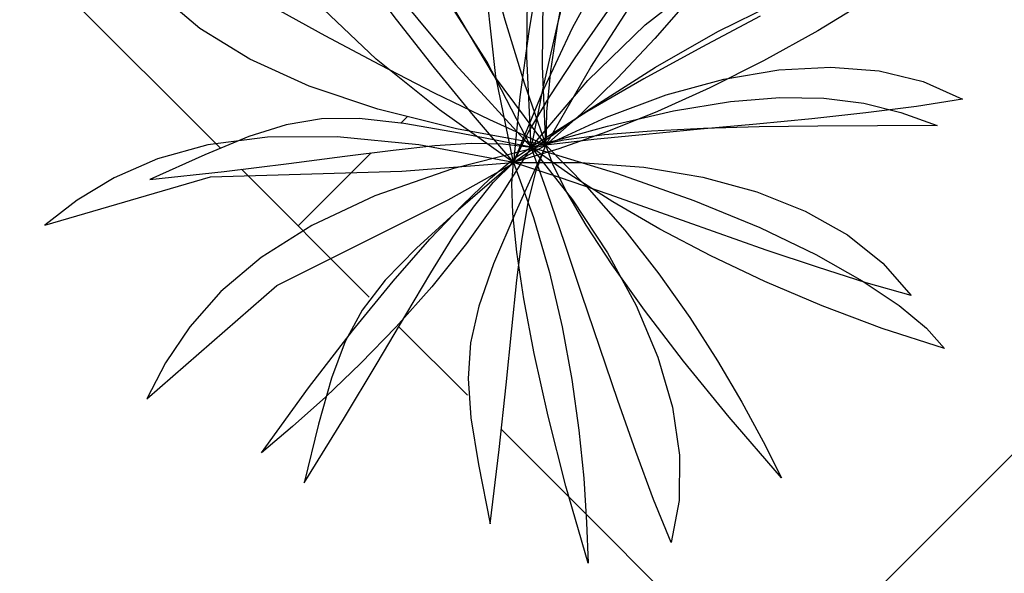
# Model space of a CAD drawing. Units: inches. Extents: x 3590 to 5167, y 65 to 1917.
# Tile 39 of 100: x 5035 to 5065, y 1340 to 1357. Entities that reach past the tile are written whole.
import ezdxf

# ---------------------------------------------------------------- set-up
doc = ezdxf.new("R2010")
doc.units = ezdxf.units.IN
doc.layers.add('A-FLOR-PATT', color=8, linetype='Continuous', lineweight=13)
doc.layers.add('L-PLNT', color=94, linetype='Continuous', lineweight=18)
doc.layers.add('DIENHOA', color=3, linetype='Continuous')

# ---------------------------------------------------------------- blocks, each defined once
blk = doc.blocks.new('Cay03_mb')
at = {"layer": 'DIENHOA'}
for p, q in [((-240.2, 277.8), (-88.4, 94.9)), ((55.7, 216.3), (37.3, 142.1)), ((0.2, 104.9), (1.6, 205.7)), ((147, 144.1), (218.5, 199.8)), ((-49.6, 98.5), (-104.2, 184.4)), ((290.2, 154.9), (217.4, 116.6)), ((37.3, 142.1), (20.5, 67.6)), ((75.9, 75.2), (147, 144.1)), ((217.4, 116.6), (145.5, 77.3)), ((5.4, -7.8), (-49.6, 98.5)), ((5.4, -7.8), (0.2, 104.9)), ((-88.4, 94.9), (5.4, -7.8)), ((5.4, -7.8), (75.9, 75.2)), ((145.5, 77.3), (74.7, 36.1)), ((20.5, 67.6), (5.4, -7.8)), ((182.2, 37.2), (253, 48.9)), ((253, 48.9), (314.6, 54.1)), ((314.6, 54.1), (369.2, 53.3)), ((369.2, 53.3), (418.6, 46.8)), ((100.3, 18.4), (182.2, 37.2)), ((418.6, 46.8), (464.9, 35.2)), ((-254.7, 27.4), (-298.6, 20.1)), ((-208, 27.8), (-254.7, 27.4)), ((-152.7, 21.7), (-208, 27.8)), ((74.7, 36.1), (5.4, -7.8)), ((464.9, 35.2), (510, 19)), ((-298.6, 20.1), (-345, 5.4)), ((-83.4, 9.7), (-152.7, 21.7)), ((5.4, -7.8), (100.3, 18.4)), ((219.6, 15.4), (155, 12.2)), ((289, 17.4), (219.6, 15.4)), ((361.6, 18.5), (289, 17.4)), ((435.8, 18.9), (361.6, 18.5)), ((510, 19), (435.8, 18.9)), ((-345, 5.4), (-399.6, -17.1)), ((5.4, -7.8), (-83.4, 9.7)), ((46.3, 0.9), (5.4, -7.8)), ((96.7, 7.5), (46.3, 0.9)), ((155, 12.2), (96.7, 7.5)), ((-225.8, -18.9), (-165.8, -11.3)), ((-165.8, -11.3), (-114, -5.7)), ((-114, -5.7), (-69, -2.9)), ((-69, -2.9), (-29.6, -3.4)), ((5.4, -7.8), (-33.2, -69.5)), ((-29.6, -3.4), (5.4, -7.8)), ((-16.5, -22.4), (5.4, -7.8)), ((5.4, -7.8), (56.8, -73.3)), ((25.9, -64.4), (5.4, -7.8)), ((5.4, -7.8), (112.8, -40.3)), ((53.5, -41.6), (5.4, -7.8)), ((-399.6, -17.1), (-468, -47.9)), ((-295.3, -27.9), (-225.8, -18.9)), ((-45.1, -46.3), (-16.5, -22.4)), ((-375.6, -37.8), (-295.3, -27.9)), ((-468, -47.9), (-375.6, -37.8)), ((-79.8, -79.6), (-45.1, -46.3)), ((107, -75.7), (53.5, -41.6)), ((112.8, -40.3), (207.5, -73.8)), ((-33.2, -69.5), (-74.6, -127.3)), ((47, -125.9), (25.9, -64.4)), ((56.8, -73.3), (100.4, -139.1)), ((-120.2, -122.1), (-79.8, -79.6)), ((165.5, -109.6), (107, -75.7)), ((207.5, -73.8), (289.5, -107.6)), ((228.7, -142.8), (165.5, -109.6)), ((289.5, -107.6), (359.3, -141.1)), ((-165.9, -174.1), (-120.2, -122.1)), ((-74.6, -127.3), (-117.8, -181.1)), ((68.7, -190.6), (47, -125.9)), ((100.4, -139.1), (135.9, -204.3)), ((296, -174.7), (228.7, -142.8)), ((359.3, -141.1), (416.9, -173.5)), ((-216.3, -235.6), (-165.9, -174.1)), ((-117.8, -181.1), (-162.1, -230.9)), ((367.1, -204.8), (296, -174.7)), ((416.9, -173.5), (462.6, -204.2)), ((90.8, -256.6), (68.7, -190.6)), ((135.9, -204.3), (162.8, -268.3)), ((441.6, -232.7), (367.1, -204.8)), ((462.6, -204.2), (496.5, -232.5)), ((-162.1, -230.9), (-206.3, -276.5)), ((-271, -306.6), (-216.3, -235.6)), ((518.9, -257.7), (441.6, -232.7)), ((496.5, -232.5), (518.9, -257.7)), ((113.1, -322.2), (90.8, -256.6)), ((162.8, -268.3), (181, -330.4)), ((-206.3, -276.5), (-249.6, -317.8)), ((-329.5, -387.1), (-271, -306.6)), ((-249.6, -317.8), (-291, -354.7)), ((135.4, -385.6), (113.1, -322.2)), ((181, -330.4), (190, -390)), ((-291, -354.7), (-329.5, -387.1)), ((157.6, -445), (135.4, -385.6)), ((190, -390), (189.6, -446.3)), ((179.5, -498.7), (157.6, -445)), ((189.6, -446.3), (179.5, -498.7))]:
    blk.add_line(p, q, dxfattribs=at)
for points in [[(23.7, -5.4), (-41, 82.2), (-91.8, 167.1), (-129.7, 249.5), (-155.6, 329.6), (-170.2, 407.8), (-174.7, 484.2), (-169.8, 559.3), (-156.5, 633.1)], [(-156.5, 633.1), (-132.5, 551.3), (-110.5, 470), (-89.8, 389.2), (-69.6, 309), (-49, 229.4), (-27.1, 150.4), (-3.2, 72.1), (23.7, -5.4)], [(-16.4, -26.7), (-38.3, 80), (-48.9, 178.3), (-48.7, 269), (-38.5, 352.6), (-19.1, 429.7), (9, 501), (44.9, 567.1), (87.9, 628.5)], [(87.9, 628.5), (75.5, 544.2), (61.3, 461.2), (46.1, 379.1), (30.8, 297.8), (16.1, 216.9), (2.9, 136), (-8.3, 54.9), (-16.4, -26.7)], [(23.7, -5.4), (19.8, 93), (20.3, 177), (25, 248.5), (34, 309.8), (47.3, 362.7), (64.9, 409.3), (86.8, 451.7), (112.9, 491.9)], [(112.9, 491.9), (96, 419.7), (79.5, 347.4), (63.9, 276.5), (50, 208.4), (38.4, 144.8), (29.7, 86.9), (24.6, 36.3), (23.7, -5.4)], [(-395.6, 473.7), (-347.5, 405.6), (-300.6, 339.5), (-254.3, 275.1), (-208.3, 212.3), (-161.9, 150.9), (-114.8, 90.7), (-66.5, 31.6), (-16.4, -26.7)], [(-16.4, -26.7), (-108.3, 38.6), (-186.9, 101.7), (-252.4, 163.5), (-305.1, 224.4), (-345.4, 285.2), (-373.7, 346.6), (-390.4, 409.2), (-395.6, 473.7)], [(384.3, 437.5), (342.2, 367.8), (298.1, 301.7), (252.6, 239.4), (206.1, 181.1), (159.4, 127.2), (113, 78), (67.6, 33.6), (23.7, -5.4)], [(23.7, -5.4), (79.9, 91.7), (134.1, 176.2), (185.8, 248.4), (234.3, 308.7), (279, 357.3), (319.3, 394.8), (354.6, 421.4), (384.3, 437.5)], [(273.2, 387.3), (227.6, 328.8), (182.3, 270.1), (138.4, 212.3), (97.2, 156.4), (60, 103.4), (27.8, 54.6), (1.9, 10.8), (-16.4, -26.7)], [(-16.4, -26.7), (21.4, 64.2), (57, 140.3), (91.4, 203.3), (125.2, 255.1), (159.5, 297.5), (195, 332.5), (232.7, 361.8), (273.2, 387.3)], [(-530.5, 289.7), (-458.3, 248.1), (-387.9, 207.8), (-318.9, 168.7), (-250.8, 131.1), (-182.9, 94.8), (-114.9, 59.9), (-46.2, 26.5), (23.7, -5.4)], [(23.7, -5.4), (-87.2, 15.2), (-185, 39.6), (-270.3, 68.2), (-343.7, 101.4), (-405.9, 139.7), (-457.3, 183.5), (-498.7, 233.4), (-530.5, 289.7)], [(496.7, 224), (429.4, 178.4), (361.6, 136.9), (294.1, 99.5), (227.5, 66.1), (162.4, 36.7), (99.7, 11.5), (39.8, -9.7), (-16.4, -26.7)], [(-16.4, -26.7), (75.4, 37.9), (160.1, 91.8), (237.3, 135.7), (306.6, 170), (367.6, 195.4), (419.9, 212.5), (463.1, 221.9), (496.7, 224)], [(23.7, -5.4), (99.3, 29.7), (173.2, 57.1), (244.8, 76.7), (313.3, 88.3), (377.9, 91.8), (437.9, 87), (492.7, 73.8), (541.4, 52)], [(541.4, 52), (484.1, 42.9), (421.2, 34.8), (354.4, 27.6), (285.4, 20.9), (216.1, 14.5), (148.2, 8.1), (83.5, 1.6), (23.7, -5.4)], [(-16.4, -26.7), (-134, -4.7), (-235.3, 5.3), (-322, 4.7), (-395.9, -5), (-458.7, -22.3), (-512.3, -45.7), (-558.2, -73.6), (-598.4, -104.7)], [(-471.9, -320.3), (-310.5, -179.3), (-97.7, -73.3), (23.7, -5.4)], [(23.7, -5.4), (-92.3, -34.8), (-188.4, -68.2), (-266.9, -105.1), (-329.9, -144.9), (-379.7, -187), (-418.5, -230.7), (-448.5, -275.3), (-471.9, -320.3)], [(23.7, -5.4), (-13.6, -87.9), (-41.1, -152.6), (-59.6, -205), (-69.9, -250.7), (-72.8, -295), (-69.2, -343.6), (-59.7, -401.9), (-45.3, -475.5)], [(-45.3, -475.5), (-34.1, -383.2), (-25.4, -302.8), (-18.3, -233.1), (-12, -172.9), (-5.6, -121.2), (2, -76.8), (11.4, -38.5), (23.7, -5.4)], [(316.5, -418.1), (251.4, -342.8), (194.8, -273.3), (146.5, -210.2), (106.3, -153.8), (74.1, -104.7), (49.7, -63.4), (32.9, -30.1), (23.7, -5.4)], [(23.7, -5.4), (74.9, -57.1), (121.8, -110.6), (164.3, -165), (202.7, -219.4), (237, -272.9), (267.3, -324.5), (293.7, -373.2), (316.5, -418.1)], [(-598.4, -104.7), (-392.7, -44.4), (-155, -37.4), (-16.4, -26.7)], [(-276.2, -424.4), (-227.3, -345.4), (-185.7, -276.1), (-150, -215.7), (-119.1, -163.8), (-91.5, -119.5), (-66, -82.3), (-41.4, -51.6), (-16.4, -26.7)], [(-16.4, -26.7), (-84.9, -86), (-137, -133.1), (-175.8, -173), (-204.3, -210), (-225.5, -249.1), (-242.5, -294.7), (-258.4, -351.6), (-276.2, -424.4)], [(76.2, -524.2), (48.8, -428.5), (26.6, -341.7), (9.2, -264.1), (-3.6, -196.1), (-12.3, -138), (-17.1, -90.2), (-18.3, -53), (-16.4, -26.7)], [(-16.4, -26.7), (66.9, -26.6), (145.6, -32.7), (218.8, -44.9), (285.8, -63.1), (345.9, -87.1), (398.4, -116.6), (442.6, -151.6), (477.6, -191.8)], [(477.6, -191.8), (421.8, -176), (361.3, -156.9), (297.6, -135.5), (232.2, -112.6), (166.6, -89.4), (102.3, -66.6), (40.8, -45.4), (-16.4, -26.7)], [(-16.4, -26.7), (8.5, -95.1), (28.5, -163.3), (44.3, -230.6), (56.3, -296.1), (65, -359), (70.9, -418.5), (74.5, -473.9), (76.2, -524.2)]]:
    blk.add_lwpolyline(points, dxfattribs=at)

msp = doc.modelspace()

# ---------------------------------------------------------------- hatches: boundary and pattern name
at = {"layer": 'A-FLOR-PATT', "transparency": 33554687}
h = msp.add_hatch(dxfattribs=at)
h.set_pattern_fill('AR-HBONE', color=256, scale=0.2)
h.set_pattern_definition([(45, (-588.972, 0), (0, 28.73682), [60.96, -20.32]), (135, (-574.604, 14.368), (3e-15, 28.73682), [60.96, -20.32])])
h.paths.add_polyline_path([(5071.274, 1796.999), (4933.274, 1796.999), (4933.274, 1753.999), (4962.774, 1753.999, -0.414214), (4928.774, 1719.999), (4933.274, 1718.999), (4933.274, 1334.999), (5071.274, 1334.999)])
h.paths.add_polyline_path([(4951.78, 1521.077), (4951.715, 1521.04), (4951.563, 1520.895)], flags=16)
h.paths.add_polyline_path([(4952.267, 1521.376), (4952.198, 1521.371), (4952.198, 1521.356)], flags=0)
h.paths.add_polyline_path([(4967.051, 1529.728), (4965.231, 1528.694), (4963.411, 1527.714), (4961.756, 1526.851), (4963.589, 1527.449), (4964.036, 1527.478), (4962.975, 1527.249), (4961.76, 1526.852), (4959.792, 1525.834), (4958.005, 1524.895), (4956.24, 1523.93), (4954.504, 1522.919), (4954.129, 1522.682), (4953.361, 1521.997), (4953.366, 1521.998), (4953.605, 1522.064), (4955.106, 1522.761), (4956.921, 1523.434), (4958.678, 1523.915), (4960.358, 1524.2), (4961.945, 1524.286), (4964.171, 1524.108), (4965.958, 1523.309), (4963.863, 1522.976), (4965.187, 1522.499), (4963.366, 1522.497), (4961.545, 1522.487), (4959.764, 1522.461), (4958.304, 1522.419), (4957.974, 1522.388), (4956.307, 1522.232), (4954.718, 1522.071), (4953.251, 1521.899), (4953.525, 1521.623), (4954.331, 1521.379), (4956.243, 1521.23), (4958.039, 1520.93), (4959.684, 1520.483), (4961.16, 1519.896), (4963.107, 1518.8), (4964.393, 1517.325), (4962.973, 1517.726), (4964.558, 1516.661), (4965.407, 1515.708), (4963.507, 1516.322), (4961.68, 1517.005), (4959.935, 1517.745), (4958.282, 1518.528), (4956.732, 1519.343), (4955.295, 1520.175), (4954.672, 1520.572), (4954.513, 1520.627), (4955.658, 1519.318), (4956.703, 1517.982), (4957.644, 1516.647), (4958.485, 1515.334), (4959.55, 1513.524), (4960.438, 1511.769), (4958.841, 1513.62), (4957.452, 1515.325), (4955.819, 1517.459), (4956.665, 1515.448), (4957.111, 1513.923), (4957.447, 1511.714), (4957.076, 1509.793), (4956.538, 1511.11), (4955.992, 1512.569), (4955.444, 1514.125), (4954.898, 1515.735), (4954.357, 1517.356), (4953.824, 1518.943), (4953.305, 1520.452), (4953.065, 1521.116), (4952.971, 1521.146), (4952.949, 1521.086), (4952.73, 1520.199), (4953.37, 1518.024), (4953.757, 1516.373), (4954.051, 1514.765), (4954.264, 1513.221), (4954.471, 1511.131), (4954.497, 1510.402), (4954.409, 1511.76), (4954.264, 1513.221), (4954.051, 1514.765), (4953.757, 1516.373), (4953.37, 1518.024), (4952.877, 1519.698), (4952.716, 1520.141), (4952.533, 1519.059), (4952.374, 1517.789), (4952.219, 1516.312), (4952.046, 1514.6), (4951.833, 1512.626), (4951.557, 1510.363), (4951.203, 1512.168), (4950.852, 1514.339), (4950.985, 1516.376), (4951.66, 1518.286), (4952.593, 1520.481), (4952.357, 1521.13), (4951.855, 1520.328), (4950.839, 1518.908), (4949.777, 1517.587), (4948.916, 1516.617), (4948.111, 1515.256), (4947.089, 1513.554), (4945.889, 1511.615), (4946.326, 1513.402), (4946.562, 1514.249), (4945.528, 1513.327), (4944.581, 1512.531), (4946.018, 1514.508), (4947.204, 1516.048), (4947.893, 1517.313), (4949.307, 1518.764), (4950.414, 1519.767), (4950.451, 1519.806), (4952.267, 1521.376), (4951.645, 1521.493), (4950.404, 1521.18), (4948.044, 1520.359), (4946.119, 1519.452), (4944.572, 1518.475), (4943.35, 1517.443), (4941.997, 1515.92), (4941.661, 1515.275), (4942.813, 1516.99), (4944.572, 1518.475), (4946.119, 1519.452), (4948.044, 1520.359), (4950.404, 1521.18), (4951.645, 1521.493), (4949.647, 1521.868), (4948.6, 1521.756), (4947.126, 1521.57), (4945.42, 1521.348), (4943.45, 1521.105), (4941.183, 1520.856), (4942.86, 1521.613), (4943.873, 1522.03), (4942.952, 1521.909), (4941.41, 1521.485), (4939.543, 1520.67), (4938.968, 1520.226), (4940.733, 1521.299), (4942.952, 1521.909), (4943.702, 1522.008), (4945.894, 1522.7), (4947.565, 1522.714), (4948.921, 1522.566), (4951.131, 1522.183), (4950.971, 1522.297), (4948.129, 1523.006), (4946.035, 1523.707), (4944.232, 1524.521), (4942.707, 1525.461), (4941.444, 1526.537), (4940.43, 1527.761), (4939.649, 1529.143), (4941.421, 1528.122), (4943.147, 1527.132), (4944.841, 1526.175), (4946.514, 1525.25), (4948.179, 1524.359), (4948.365, 1524.263), (4946.475, 1526.045), (4945.181, 1527.54), (4944.19, 1529.033), (4943.496, 1530.54), (4943.278, 1531.36), (4942.498, 1531.919), (4943.114, 1531.762), (4942.959, 1533.659), (4944.14, 1531.989), (4944.612, 1531.323), (4946.202, 1530.463), (4947.486, 1529.509), (4948.79, 1528.226), (4950.368, 1526.237), (4949.485, 1528.155), (4948.851, 1530.123), (4948.491, 1532.041), (4948.381, 1533.918), (4948.501, 1535.76), (4948.827, 1537.573), (4949.418, 1535.565), (4949.957, 1533.569), (4950.464, 1531.586), (4950.961, 1529.617), (4951.391, 1527.954), (4951.724, 1530.687), (4952.201, 1532.58), (4952.889, 1534.33), (4953.77, 1535.951), (4954.827, 1537.46), (4954.521, 1535.39), (4954.273, 1533.937), (4955.58, 1535.663), (4956.748, 1536.739), (4956.159, 1534.78), (4955.589, 1532.873), (4955.043, 1531.006), (4954.525, 1529.166), (4954.038, 1527.341), (4953.638, 1525.733), (4953.611, 1525.586), (4953.398, 1524.166), (4953.382, 1524.009), (4954.07, 1525.476), (4954.912, 1527.022), (4956.136, 1528.894), (4957.847, 1530.577), (4959.376, 1531.54), (4958.256, 1530.104), (4957.143, 1528.663), (4956.066, 1527.243), (4955.056, 1525.871), (4954.141, 1524.571), (4953.352, 1523.372), (4953.311, 1523.303), (4953.273, 1522.925), (4953.261, 1522.382), (4954.103, 1523.373), (4954.63, 1524.284), (4955.961, 1526.358), (4957.23, 1528.13), (4958.421, 1529.609), (4960.037, 1531.368), (4961.374, 1532.375), (4962.101, 1532.77), (4961.07, 1531.061), (4959.987, 1529.438), (4958.869, 1527.908), (4958.15, 1527.007), (4959.803, 1528.003), (4961.589, 1528.793), (4963.391, 1529.328), (4965.211, 1529.632)], flags=16)
h.paths.add_polyline_path([(4962.944, 1523.182), (4961.107, 1523.422), (4960.392, 1523.362), (4962.35, 1523.331)], flags=0)
h.paths.add_polyline_path([(5049.541, 1584.551), (5049.476, 1584.515), (5049.325, 1584.37)], flags=16)
h.paths.add_polyline_path([(5050.028, 1584.851), (5049.959, 1584.845), (5049.959, 1584.83)], flags=0)
h.paths.add_polyline_path([(5042.333, 1581.949), (5043.88, 1582.926), (5045.806, 1583.833), (5048.165, 1584.654), (5049.406, 1584.967), (5047.408, 1585.342), (5046.361, 1585.231), (5044.888, 1585.044), (5043.181, 1584.822), (5041.211, 1584.579), (5038.944, 1584.33), (5040.622, 1585.087), (5041.634, 1585.504), (5040.713, 1585.383), (5039.171, 1584.959), (5037.304, 1584.144), (5036.729, 1583.7), (5038.494, 1584.773), (5040.713, 1585.383), (5041.463, 1585.482), (5043.655, 1586.174), (5045.326, 1586.188), (5046.682, 1586.04), (5048.893, 1585.657), (5048.732, 1585.771), (5045.891, 1586.48), (5043.796, 1587.181), (5041.994, 1587.996), (5040.468, 1588.935), (5039.205, 1590.011), (5038.191, 1591.235), (5037.41, 1592.617), (5039.182, 1591.596), (5040.909, 1590.607), (5042.602, 1589.649), (5044.275, 1588.724), (5045.94, 1587.833), (5046.126, 1587.738), (5044.237, 1589.519), (5042.942, 1591.015), (5041.952, 1592.508), (5041.257, 1594.014), (5041.039, 1594.834), (5040.26, 1595.393), (5040.875, 1595.237), (5040.721, 1597.133), (5041.901, 1595.463), (5042.373, 1594.798), (5043.963, 1593.938), (5045.247, 1592.983), (5046.552, 1591.701), (5048.129, 1589.712), (5047.247, 1591.63), (5046.613, 1593.597), (5046.252, 1595.515), (5046.142, 1597.392), (5046.262, 1599.234), (5046.588, 1601.047), (5047.179, 1599.039), (5047.718, 1597.043), (5048.225, 1595.06), (5048.722, 1593.091), (5049.152, 1591.429), (5049.485, 1594.161), (5049.962, 1596.054), (5050.65, 1597.804), (5051.532, 1599.425), (5052.589, 1600.934), (5052.283, 1598.864), (5052.034, 1597.411), (5053.341, 1599.137), (5054.509, 1600.213), (5053.92, 1598.254), (5053.35, 1596.348), (5052.805, 1594.48), (5052.286, 1592.64), (5051.799, 1590.815), (5051.4, 1589.207), (5051.373, 1589.06), (5051.159, 1587.64), (5051.143, 1587.483), (5051.831, 1588.95), (5052.673, 1590.496), (5053.898, 1592.368), (5055.608, 1594.051), (5057.137, 1595.014), (5056.017, 1593.578), (5054.904, 1592.137), (5053.828, 1590.717), (5052.817, 1589.345), (5051.902, 1588.046), (5051.113, 1586.846), (5051.072, 1586.777), (5051.034, 1586.399), (5051.022, 1585.856), (5051.864, 1586.847), (5052.391, 1587.758), (5053.723, 1589.832), (5054.991, 1591.604), (5056.182, 1593.083), (5057.798, 1594.842), (5059.135, 1595.849), (5059.863, 1596.244), (5058.831, 1594.535), (5057.749, 1592.912), (5056.63, 1591.382), (5055.912, 1590.482), (5057.564, 1591.477), (5059.35, 1592.267), (5061.152, 1592.802), (5062.972, 1593.106), (5064.812, 1593.203), (5062.992, 1592.169), (5061.172, 1591.188), (5059.518, 1590.325), (5061.35, 1590.924), (5061.797, 1590.952), (5060.737, 1590.723), (5059.521, 1590.326), (5057.553, 1589.308), (5055.766, 1588.369), (5054.002, 1587.404), (5052.265, 1586.393), (5051.891, 1586.156), (5051.122, 1585.471), (5051.127, 1585.472), (5051.366, 1585.538), (5052.867, 1586.235), (5054.682, 1586.908), (5056.439, 1587.389), (5058.12, 1587.675), (5059.706, 1587.76), (5061.933, 1587.583), (5063.719, 1586.783), (5061.624, 1586.45), (5062.949, 1585.973), (5061.127, 1585.971), (5059.307, 1585.961), (5057.525, 1585.935), (5056.065, 1585.893), (5055.735, 1585.862), (5054.068, 1585.707), (5052.479, 1585.546), (5051.012, 1585.373), (5051.286, 1585.097), (5052.092, 1584.853), (5054.004, 1584.704), (5055.8, 1584.404), (5057.446, 1583.958), (5058.921, 1583.37), (5060.868, 1582.274), (5062.154, 1580.799), (5060.734, 1581.2), (5062.32, 1580.135), (5063.168, 1579.182), (5061.269, 1579.796), (5059.441, 1580.479), (5057.696, 1581.219), (5056.043, 1582.003), (5054.493, 1582.817), (5053.057, 1583.649), (5052.433, 1584.047), (5052.274, 1584.101), (5053.42, 1582.793), (5054.464, 1581.457), (5055.405, 1580.121), (5056.247, 1578.809), (5057.311, 1576.998), (5058.199, 1575.244), (5056.602, 1577.094), (5055.213, 1578.799), (5053.58, 1580.933), (5054.427, 1578.922), (5054.872, 1577.397), (5055.208, 1575.189), (5054.838, 1573.267), (5054.299, 1574.584), (5053.754, 1576.043), (5053.206, 1577.599), (5052.659, 1579.209), (5052.118, 1580.83), (5051.585, 1582.417), (5051.066, 1583.927), (5050.826, 1584.59), (5050.733, 1584.62), (5050.711, 1584.561), (5050.491, 1583.673), (5051.131, 1581.498), (5051.518, 1579.847), (5051.813, 1578.24), (5052.026, 1576.695), (5052.233, 1574.605), (5052.258, 1573.876), (5052.17, 1575.234), (5052.026, 1576.695), (5051.813, 1578.24), (5051.518, 1579.847), (5051.131, 1581.498), (5050.638, 1583.172), (5050.477, 1583.615), (5050.294, 1582.533), (5050.136, 1581.263), (5049.981, 1579.786), (5049.807, 1578.074), (5049.594, 1576.1), (5049.318, 1573.837), (5048.965, 1575.642), (5048.613, 1577.813), (5048.747, 1579.85), (5049.421, 1581.76), (5050.354, 1583.955), (5050.118, 1584.604), (5049.616, 1583.802), (5048.6, 1582.382), (5047.538, 1581.061), (5046.677, 1580.091), (5045.872, 1578.73), (5044.85, 1577.028), (5043.651, 1575.089), (5044.087, 1576.877), (5044.324, 1577.723), (5043.289, 1576.801), (5042.342, 1576.005), (5043.779, 1577.982), (5044.966, 1579.522), (5045.655, 1580.787), (5047.068, 1582.239), (5048.175, 1583.241), (5048.213, 1583.28), (5050.028, 1584.851), (5049.406, 1584.967), (5048.165, 1584.654), (5045.806, 1583.833), (5043.88, 1582.926), (5042.333, 1581.949), (5041.111, 1580.917), (5039.758, 1579.394), (5039.423, 1578.749), (5040.575, 1580.464)], flags=16)
h.paths.add_polyline_path([(4954.799, 1533.12), (4954.262, 1532.079), (4953.831, 1530.935), (4953.505, 1529.636), (4953.283, 1528.133), (4953.167, 1526.376), (4953.156, 1524.315), (4953.277, 1521.236), (4952.802, 1521.842), (4951.557, 1521.998), (4950.976, 1521.961), (4952.661, 1521.941), (4952.802, 1521.842), (4953.152, 1523.593), (4953.167, 1526.376), (4953.283, 1528.133), (4953.609, 1530.346), (4954.456, 1532.592)], flags=0)
h.paths.add_polyline_path([(5050.563, 1585.316), (5049.318, 1585.472), (5048.737, 1585.435), (5050.422, 1585.415), (5050.563, 1585.316), (5050.914, 1587.067), (5050.928, 1589.851), (5051.045, 1591.607), (5051.371, 1593.82), (5052.217, 1596.066), (5052.56, 1596.594), (5052.024, 1595.554), (5051.592, 1594.409), (5051.266, 1593.11), (5051.045, 1591.607), (5050.928, 1589.851), (5050.918, 1587.789), (5051.038, 1584.71)], flags=0)
h.paths.add_polyline_path([(5058.153, 1586.836), (5060.111, 1586.805), (5060.705, 1586.656), (5058.868, 1586.896)], flags=0)
h.paths.add_polyline_path([(5049.541, 1430.936), (5049.476, 1430.9), (5049.325, 1430.755)], flags=16)
h.paths.add_polyline_path([(5050.028, 1431.236), (5049.959, 1431.231), (5049.959, 1431.215)], flags=0)
h.paths.add_polyline_path([(5046.588, 1447.432), (5047.179, 1445.425), (5047.718, 1443.429), (5048.225, 1441.446), (5048.722, 1439.476), (5049.152, 1437.814), (5049.485, 1440.546), (5049.962, 1442.439), (5050.65, 1444.189), (5051.532, 1445.811), (5052.589, 1447.319), (5052.283, 1445.249), (5052.034, 1443.796), (5053.341, 1445.522), (5054.509, 1446.598), (5053.92, 1444.64), (5053.35, 1442.733), (5052.805, 1440.865), (5052.286, 1439.025), (5051.799, 1437.201), (5051.4, 1435.592), (5051.373, 1435.445), (5051.159, 1434.025), (5051.143, 1433.868), (5051.831, 1435.335), (5052.673, 1436.881), (5053.898, 1438.753), (5055.608, 1440.436), (5057.137, 1441.4), (5056.017, 1439.963), (5054.904, 1438.522), (5053.828, 1437.102), (5052.817, 1435.73), (5051.902, 1434.431), (5051.113, 1433.231), (5051.072, 1433.162), (5051.034, 1432.784), (5051.022, 1432.242), (5051.864, 1433.232), (5052.391, 1434.143), (5053.723, 1436.217), (5054.991, 1437.989), (5056.182, 1439.468), (5057.798, 1441.227), (5059.135, 1442.235), (5059.863, 1442.629), (5058.831, 1440.921), (5057.749, 1439.298), (5056.63, 1437.767), (5055.912, 1436.867), (5057.564, 1437.863), (5059.35, 1438.652), (5061.152, 1439.187), (5062.972, 1439.491), (5064.812, 1439.588), (5062.992, 1438.554), (5061.172, 1437.573), (5059.518, 1436.71), (5061.35, 1437.309), (5061.797, 1437.337), (5060.737, 1437.108), (5059.521, 1436.711), (5057.553, 1435.693), (5055.766, 1434.754), (5054.002, 1433.789), (5052.265, 1432.778), (5051.891, 1432.541), (5051.122, 1431.856), (5051.127, 1431.857), (5051.366, 1431.923), (5052.867, 1432.62), (5054.682, 1433.293), (5056.439, 1433.775), (5058.12, 1434.06), (5059.706, 1434.145), (5061.933, 1433.968), (5063.719, 1433.168), (5061.624, 1432.835), (5062.949, 1432.358), (5061.127, 1432.357), (5059.307, 1432.346), (5057.525, 1432.32), (5056.065, 1432.278), (5055.735, 1432.248), (5054.068, 1432.092), (5052.479, 1431.931), (5051.012, 1431.759), (5051.286, 1431.482), (5052.092, 1431.238), (5054.004, 1431.089), (5055.8, 1430.789), (5057.446, 1430.343), (5058.921, 1429.755), (5060.868, 1428.66), (5062.154, 1427.185), (5060.734, 1427.585), (5062.32, 1426.52), (5063.168, 1425.567), (5061.269, 1426.181), (5059.441, 1426.865), (5057.696, 1427.604), (5056.043, 1428.388), (5054.493, 1429.202), (5053.057, 1430.034), (5052.433, 1430.432), (5052.274, 1430.487), (5053.42, 1429.178), (5054.464, 1427.842), (5055.405, 1426.506), (5056.247, 1425.194), (5057.311, 1423.383), (5058.199, 1421.629), (5056.602, 1423.479), (5055.213, 1425.184), (5053.58, 1427.318), (5054.427, 1425.307), (5054.872, 1423.782), (5055.208, 1421.574), (5054.838, 1419.652), (5054.299, 1420.97), (5053.754, 1422.428), (5053.206, 1423.984), (5052.659, 1425.595), (5052.118, 1427.215), (5051.585, 1428.802), (5051.066, 1430.312), (5050.826, 1430.975), (5050.733, 1431.005), (5050.711, 1430.946), (5050.491, 1430.058), (5051.131, 1427.883), (5051.518, 1426.232), (5051.813, 1424.625), (5052.026, 1423.081), (5052.233, 1420.991), (5052.258, 1420.261), (5052.17, 1421.619), (5052.026, 1423.081), (5051.813, 1424.625), (5051.518, 1426.232), (5051.131, 1427.883), (5050.638, 1429.558), (5050.477, 1430.001), (5050.294, 1428.918), (5050.136, 1427.648), (5049.981, 1426.171), (5049.807, 1424.459), (5049.594, 1422.485), (5049.318, 1420.222), (5048.965, 1422.028), (5048.613, 1424.199), (5048.747, 1426.235), (5049.421, 1428.146), (5050.354, 1430.34), (5050.118, 1430.989), (5049.616, 1430.187), (5048.6, 1428.768), (5047.538, 1427.446), (5046.677, 1426.477), (5045.872, 1425.116), (5044.85, 1423.413), (5043.651, 1421.474), (5044.087, 1423.262), (5044.324, 1424.109), (5043.289, 1423.186), (5042.342, 1422.391), (5043.779, 1424.368), (5044.966, 1425.907), (5045.655, 1427.173), (5047.068, 1428.624), (5048.175, 1429.627), (5048.213, 1429.666), (5050.028, 1431.236), (5049.406, 1431.353), (5048.165, 1431.039), (5045.806, 1430.218), (5043.88, 1429.311), (5042.333, 1428.334), (5041.111, 1427.302), (5039.758, 1425.779), (5039.423, 1425.134), (5040.575, 1426.849), (5042.333, 1428.334), (5043.88, 1429.311), (5045.806, 1430.218), (5048.165, 1431.039), (5049.406, 1431.353), (5047.408, 1431.727), (5046.361, 1431.616), (5044.888, 1431.429), (5043.181, 1431.207), (5041.211, 1430.964), (5038.944, 1430.715), (5040.622, 1431.472), (5041.634, 1431.89), (5040.713, 1431.769), (5039.171, 1431.345), (5037.304, 1430.53), (5036.729, 1430.085), (5038.494, 1431.158), (5040.713, 1431.769), (5041.463, 1431.867), (5043.655, 1432.559), (5045.326, 1432.573), (5046.682, 1432.425), (5048.893, 1432.042), (5048.732, 1432.156), (5045.891, 1432.865), (5043.796, 1433.566), (5041.994, 1434.381), (5040.468, 1435.321), (5039.205, 1436.396), (5038.191, 1437.62), (5037.41, 1439.002), (5039.182, 1437.982), (5040.909, 1436.992), (5042.602, 1436.034), (5044.275, 1435.109), (5045.94, 1434.218), (5046.126, 1434.123), (5044.237, 1435.904), (5042.942, 1437.4), (5041.952, 1438.893), (5041.257, 1440.399), (5041.039, 1441.219), (5040.26, 1441.778), (5040.875, 1441.622), (5040.721, 1443.518), (5041.901, 1441.848), (5042.373, 1441.183), (5043.963, 1440.323), (5045.247, 1439.369), (5046.552, 1438.086), (5048.129, 1436.097), (5047.247, 1438.015), (5046.613, 1439.982), (5046.252, 1441.901), (5046.142, 1443.778), (5046.262, 1445.619)], flags=16)
h.paths.add_polyline_path([(5052.382, 1444.255), (5051.623, 1442.78), (5052.024, 1441.939), (5052.56, 1442.98)], flags=0)
h.paths.add_polyline_path([(5050.563, 1431.701), (5049.318, 1431.857), (5048.737, 1431.821), (5050.422, 1431.8)], flags=0)
h.paths.add_polyline_path([(5058.153, 1433.221), (5060.111, 1433.19), (5060.705, 1433.041), (5058.868, 1433.281)], flags=0)
h.paths.add_polyline_path([(5049.541, 1352.285), (5049.476, 1352.249), (5049.325, 1352.104)], flags=16)
h.paths.add_polyline_path([(5050.028, 1352.585), (5049.959, 1352.58), (5049.959, 1352.564)], flags=0)
h.paths.add_polyline_path([(5046.588, 1368.781), (5047.179, 1366.774), (5047.718, 1364.778), (5048.225, 1362.795), (5048.722, 1360.825), (5049.152, 1359.163), (5049.485, 1361.896), (5049.962, 1363.789), (5050.65, 1365.538), (5051.532, 1367.16), (5052.589, 1368.669), (5052.283, 1366.598), (5052.034, 1365.145), (5053.341, 1366.871), (5054.509, 1367.947), (5053.92, 1365.989), (5053.35, 1364.082), (5052.805, 1362.214), (5052.286, 1360.374), (5051.799, 1358.55), (5051.4, 1356.942), (5051.373, 1356.794), (5051.159, 1355.374), (5051.143, 1355.218), (5051.831, 1356.684), (5052.673, 1358.23), (5053.898, 1360.102), (5055.608, 1361.786), (5057.137, 1362.749), (5056.017, 1361.313), (5054.904, 1359.872), (5053.828, 1358.452), (5052.817, 1357.079), (5051.902, 1355.78), (5051.113, 1354.581), (5051.072, 1354.512), (5051.034, 1354.133), (5051.022, 1353.591), (5051.864, 1354.581), (5052.391, 1355.492), (5053.723, 1357.566), (5054.991, 1359.338), (5056.182, 1360.817), (5057.798, 1362.577), (5059.135, 1363.584), (5059.863, 1363.979), (5058.831, 1362.27), (5057.749, 1360.647), (5056.63, 1359.117), (5055.912, 1358.216), (5057.564, 1359.212), (5059.35, 1360.001), (5061.152, 1360.536), (5062.972, 1360.841), (5064.812, 1360.937), (5062.992, 1359.903), (5061.172, 1358.923), (5059.518, 1358.059), (5061.35, 1358.658), (5061.797, 1358.687), (5060.737, 1358.458), (5059.521, 1358.061), (5057.553, 1357.043), (5055.766, 1356.103), (5054.002, 1355.138), (5052.265, 1354.127), (5051.891, 1353.89), (5051.122, 1353.206), (5051.127, 1353.206), (5051.366, 1353.272), (5052.867, 1353.969), (5054.682, 1354.643), (5056.439, 1355.124), (5058.12, 1355.409), (5059.706, 1355.495), (5061.933, 1355.317), (5063.719, 1354.518), (5061.624, 1354.184), (5062.949, 1353.708), (5061.127, 1353.706), (5059.307, 1353.695), (5057.525, 1353.669), (5056.065, 1353.627), (5055.735, 1353.597), (5054.068, 1353.441), (5052.479, 1353.28), (5051.012, 1353.108), (5051.286, 1352.831), (5052.092, 1352.587), (5054.004, 1352.439), (5055.8, 1352.138), (5057.446, 1351.692), (5058.921, 1351.104), (5060.868, 1350.009), (5062.154, 1348.534), (5060.734, 1348.935), (5062.32, 1347.869), (5063.168, 1346.916), (5061.269, 1347.53), (5059.441, 1348.214), (5057.696, 1348.954), (5056.043, 1349.737), (5054.493, 1350.551), (5053.057, 1351.383), (5052.433, 1351.781), (5052.274, 1351.836), (5053.42, 1350.527), (5054.464, 1349.191), (5055.405, 1347.855), (5056.247, 1346.543), (5057.311, 1344.733), (5058.199, 1342.978), (5056.602, 1344.828), (5055.213, 1346.534), (5053.58, 1348.667), (5054.427, 1346.656), (5054.872, 1345.132), (5055.208, 1342.923), (5054.838, 1341.002), (5054.299, 1342.319), (5053.754, 1343.778), (5053.206, 1345.334), (5052.659, 1346.944), (5052.118, 1348.564), (5051.585, 1350.151), (5051.066, 1351.661), (5050.826, 1352.324), (5050.733, 1352.355), (5050.711, 1352.295), (5050.491, 1351.408), (5051.131, 1349.232), (5051.518, 1347.581), (5051.813, 1345.974), (5052.026, 1344.43), (5052.233, 1342.34), (5052.258, 1341.61), (5052.17, 1342.969), (5052.026, 1344.43), (5051.813, 1345.974), (5051.518, 1347.581), (5051.131, 1349.232), (5050.638, 1350.907), (5050.477, 1351.35), (5050.294, 1350.267), (5050.136, 1348.997), (5049.981, 1347.52), (5049.807, 1345.809), (5049.594, 1343.835), (5049.318, 1341.571), (5048.965, 1343.377), (5048.613, 1345.548), (5048.747, 1347.585), (5049.421, 1349.495), (5050.354, 1351.689), (5050.118, 1352.339), (5049.616, 1351.536), (5048.6, 1350.117), (5047.538, 1348.795), (5046.677, 1347.826), (5045.872, 1346.465), (5044.85, 1344.763), (5043.651, 1342.824), (5044.087, 1344.611), (5044.324, 1345.458), (5043.289, 1344.535), (5042.342, 1343.74), (5043.779, 1345.717), (5044.966, 1347.256), (5045.655, 1348.522), (5047.068, 1349.973), (5048.175, 1350.976), (5048.213, 1351.015), (5050.028, 1352.585), (5049.406, 1352.702), (5048.165, 1352.388), (5045.806, 1351.567), (5043.88, 1350.661), (5042.333, 1349.683), (5041.111, 1348.651), (5039.758, 1347.128), (5039.423, 1346.483), (5040.575, 1348.198), (5042.333, 1349.683), (5043.88, 1350.661), (5045.806, 1351.567), (5048.165, 1352.388), (5049.406, 1352.702), (5047.408, 1353.076), (5046.361, 1352.965), (5044.888, 1352.779), (5043.181, 1352.556), (5041.211, 1352.313), (5038.944, 1352.065), (5040.622, 1352.821), (5041.634, 1353.239), (5040.713, 1353.118), (5039.171, 1352.694), (5037.304, 1351.879), (5036.729, 1351.434), (5038.494, 1352.508), (5040.713, 1353.118), (5041.463, 1353.216), (5043.655, 1353.909), (5045.326, 1353.923), (5046.682, 1353.774), (5048.893, 1353.391), (5048.732, 1353.506), (5045.891, 1354.214), (5043.796, 1354.915), (5041.994, 1355.73), (5040.468, 1356.67), (5039.205, 1357.746), (5038.191, 1358.969), (5037.41, 1360.352), (5039.182, 1359.331), (5040.909, 1358.341), (5042.602, 1357.383), (5044.275, 1356.458), (5045.94, 1355.567), (5046.126, 1355.472), (5044.237, 1357.253), (5042.942, 1358.749), (5041.952, 1360.242), (5041.257, 1361.748), (5041.039, 1362.568), (5040.26, 1363.128), (5040.875, 1362.971), (5040.721, 1364.867), (5041.901, 1363.197), (5042.373, 1362.532), (5043.963, 1361.672), (5045.247, 1360.718), (5046.552, 1359.435), (5048.129, 1357.446), (5047.247, 1359.364), (5046.613, 1361.331), (5046.252, 1363.25), (5046.142, 1365.127), (5046.262, 1366.969)], flags=16)
h.paths.add_polyline_path([(5052.382, 1365.604), (5051.623, 1364.129), (5052.024, 1363.288), (5052.56, 1364.329)], flags=0)
h.paths.add_polyline_path([(4951.78, 1698.041), (4951.715, 1698.005), (4951.563, 1697.859)], flags=16)
h.paths.add_polyline_path([(4952.267, 1698.341), (4952.198, 1698.335), (4952.198, 1698.32)], flags=0)
h.paths.add_polyline_path([(4957.076, 1686.757), (4956.538, 1688.074), (4955.992, 1689.533), (4955.444, 1691.089), (4954.898, 1692.699), (4954.357, 1694.32), (4953.824, 1695.907), (4953.305, 1697.417), (4953.065, 1698.08), (4952.971, 1698.11), (4952.949, 1698.051), (4952.73, 1697.163), (4953.37, 1694.988), (4953.757, 1693.337), (4954.051, 1691.729), (4954.264, 1690.185), (4954.471, 1688.095), (4954.497, 1687.366), (4954.409, 1688.724), (4954.264, 1690.185), (4954.051, 1691.729), (4953.757, 1693.337), (4953.37, 1694.988), (4952.877, 1696.662), (4952.716, 1697.105), (4952.533, 1696.023), (4952.374, 1694.753), (4952.219, 1693.276), (4952.046, 1691.564), (4951.833, 1689.59), (4951.557, 1687.327), (4951.203, 1689.132), (4950.852, 1691.303), (4950.985, 1693.34), (4951.66, 1695.25), (4952.593, 1697.445), (4952.357, 1698.094), (4951.855, 1697.292), (4950.839, 1695.872), (4949.777, 1694.551), (4948.916, 1693.581), (4948.111, 1692.22), (4947.089, 1690.518), (4945.889, 1688.579), (4946.326, 1690.366), (4946.562, 1691.213), (4945.528, 1690.291), (4944.581, 1689.495), (4946.018, 1691.472), (4947.204, 1693.012), (4947.893, 1694.277), (4949.307, 1695.729), (4950.414, 1696.731), (4950.451, 1696.77), (4952.267, 1698.341), (4951.645, 1698.457), (4950.404, 1698.144), (4948.044, 1697.323), (4946.119, 1696.416), (4944.572, 1695.439), (4943.35, 1694.407), (4941.997, 1692.884), (4941.661, 1692.239), (4942.813, 1693.954), (4944.572, 1695.439), (4946.119, 1696.416), (4948.044, 1697.323), (4950.404, 1698.144), (4951.645, 1698.457), (4949.647, 1698.832), (4948.6, 1698.72), (4947.126, 1698.534), (4945.42, 1698.312), (4943.45, 1698.069), (4941.183, 1697.82), (4942.86, 1698.577), (4943.873, 1698.994), (4942.952, 1698.873), (4941.41, 1698.449), (4939.543, 1697.634), (4938.968, 1697.19), (4940.733, 1698.263), (4942.952, 1698.873), (4943.702, 1698.972), (4945.894, 1699.664), (4947.565, 1699.678), (4948.921, 1699.53), (4951.131, 1699.147), (4950.971, 1699.261), (4948.129, 1699.97), (4946.035, 1700.671), (4944.232, 1701.486), (4942.707, 1702.425), (4941.444, 1703.501), (4940.43, 1704.725), (4939.649, 1706.107), (4941.421, 1705.086), (4943.147, 1704.097), (4944.841, 1703.139), (4946.514, 1702.214), (4948.179, 1701.323), (4948.365, 1701.227), (4946.475, 1703.009), (4945.181, 1704.505), (4944.19, 1705.997), (4943.496, 1707.504), (4943.278, 1708.324), (4942.498, 1708.883), (4943.114, 1708.727), (4942.959, 1710.623), (4944.14, 1708.953), (4944.612, 1708.287), (4946.202, 1707.428), (4947.486, 1706.473), (4948.79, 1705.191), (4950.368, 1703.202), (4949.485, 1705.12), (4948.851, 1707.087), (4948.491, 1709.005), (4948.381, 1710.882), (4948.501, 1712.724), (4948.827, 1714.537), (4949.418, 1712.529), (4949.957, 1710.533), (4950.464, 1708.55), (4950.961, 1706.581), (4951.391, 1704.919), (4951.724, 1707.651), (4952.201, 1709.544), (4952.889, 1711.294), (4953.77, 1712.915), (4954.827, 1714.424), (4954.521, 1712.354), (4954.273, 1710.901), (4955.58, 1712.627), (4956.748, 1713.703), (4956.159, 1711.744), (4955.589, 1709.837), (4955.043, 1707.97), (4954.525, 1706.13), (4954.038, 1704.305), (4953.638, 1702.697), (4953.611, 1702.55), (4953.398, 1701.13), (4953.382, 1700.973), (4954.07, 1702.44), (4954.912, 1703.986), (4956.136, 1705.858), (4957.847, 1707.541), (4959.376, 1708.504), (4958.256, 1707.068), (4957.143, 1705.627), (4956.066, 1704.207), (4955.056, 1702.835), (4954.141, 1701.536), (4953.352, 1700.336), (4953.311, 1700.267), (4953.273, 1699.889), (4953.261, 1699.346), (4954.103, 1700.337), (4954.63, 1701.248), (4955.961, 1703.322), (4957.23, 1705.094), (4958.421, 1706.573), (4960.037, 1708.332), (4961.374, 1709.339), (4962.101, 1709.734), (4961.07, 1708.025), (4959.987, 1706.402), (4958.869, 1704.872), (4958.15, 1703.972), (4959.803, 1704.967), (4961.589, 1705.757), (4963.391, 1706.292), (4965.211, 1706.596), (4967.051, 1706.692), (4965.231, 1705.659), (4963.411, 1704.678), (4961.756, 1703.815), (4963.589, 1704.413), (4964.036, 1704.442), (4962.975, 1704.213), (4961.76, 1703.816), (4959.792, 1702.798), (4958.005, 1701.859), (4956.24, 1700.894), (4954.504, 1699.883), (4954.129, 1699.646), (4953.361, 1698.961), (4953.366, 1698.962), (4953.605, 1699.028), (4955.106, 1699.725), (4956.921, 1700.398), (4958.678, 1700.879), (4960.358, 1701.164), (4961.945, 1701.25), (4964.171, 1701.073), (4965.958, 1700.273), (4963.863, 1699.94), (4965.187, 1699.463), (4963.366, 1699.461), (4961.545, 1699.451), (4959.764, 1699.425), (4958.304, 1699.383), (4957.974, 1699.352), (4956.307, 1699.197), (4954.718, 1699.036), (4953.251, 1698.863), (4953.525, 1698.587), (4954.331, 1698.343), (4956.243, 1698.194), (4958.039, 1697.894), (4959.684, 1697.447), (4961.16, 1696.86), (4963.107, 1695.764), (4964.393, 1694.289), (4962.973, 1694.69), (4964.558, 1693.625), (4965.407, 1692.672), (4963.507, 1693.286), (4961.68, 1693.969), (4959.935, 1694.709), (4958.282, 1695.492), (4956.732, 1696.307), (4955.295, 1697.139), (4954.672, 1697.536), (4954.513, 1697.591), (4955.658, 1696.282), (4956.703, 1694.946), (4957.644, 1693.611), (4958.485, 1692.298), (4959.55, 1690.488), (4960.438, 1688.733), (4958.841, 1690.584), (4957.452, 1692.289), (4955.819, 1694.423), (4956.665, 1692.412), (4957.111, 1690.887), (4957.447, 1688.678)], flags=16)
h.paths.add_polyline_path([(5050.563, 1353.05), (5049.318, 1353.207), (5048.737, 1353.17), (5050.422, 1353.15)], flags=0)
h.paths.add_polyline_path([(4951.78, 1351.486), (4951.715, 1351.45), (4951.563, 1351.305)], flags=16)
h.paths.add_polyline_path([(4952.267, 1351.786), (4952.198, 1351.78), (4952.198, 1351.765)], flags=0)
h.paths.add_polyline_path([(4954.827, 1367.869), (4954.521, 1365.799), (4954.273, 1364.346), (4955.58, 1366.072), (4956.748, 1367.148), (4956.159, 1365.19), (4955.589, 1363.283), (4955.043, 1361.415), (4954.525, 1359.575), (4954.038, 1357.751), (4953.638, 1356.142), (4953.611, 1355.995), (4953.398, 1354.575), (4953.382, 1354.418), (4954.07, 1355.885), (4954.912, 1357.431), (4956.136, 1359.303), (4957.847, 1360.986), (4959.376, 1361.95), (4958.256, 1360.513), (4957.143, 1359.072), (4956.066, 1357.652), (4955.056, 1356.28), (4954.141, 1354.981), (4953.352, 1353.781), (4953.311, 1353.712), (4953.273, 1353.334), (4953.261, 1352.792), (4954.103, 1353.782), (4954.63, 1354.693), (4955.961, 1356.767), (4957.23, 1358.539), (4958.421, 1360.018), (4960.037, 1361.777), (4961.374, 1362.785), (4962.101, 1363.179), (4961.07, 1361.471), (4959.987, 1359.848), (4958.869, 1358.317), (4958.15, 1357.417), (4959.803, 1358.413), (4961.589, 1359.202), (4963.391, 1359.737), (4965.211, 1360.041), (4967.051, 1360.138), (4965.231, 1359.104), (4963.411, 1358.123), (4961.756, 1357.26), (4963.589, 1357.859), (4964.036, 1357.887), (4962.975, 1357.658), (4961.76, 1357.261), (4959.792, 1356.243), (4958.005, 1355.304), (4956.24, 1354.339), (4954.504, 1353.328), (4954.129, 1353.091), (4953.361, 1352.406), (4953.366, 1352.407), (4953.605, 1352.473), (4955.106, 1353.17), (4956.921, 1353.843), (4958.678, 1354.325), (4960.358, 1354.61), (4961.945, 1354.695), (4964.171, 1354.518), (4965.958, 1353.718), (4963.863, 1353.385), (4965.187, 1352.908), (4963.366, 1352.907), (4961.545, 1352.896), (4959.764, 1352.87), (4958.304, 1352.828), (4957.974, 1352.798), (4956.307, 1352.642), (4954.718, 1352.481), (4953.251, 1352.309), (4953.525, 1352.032), (4954.331, 1351.788), (4956.243, 1351.639), (4958.039, 1351.339), (4959.684, 1350.893), (4961.16, 1350.305), (4963.107, 1349.21), (4964.393, 1347.735), (4962.973, 1348.135), (4964.558, 1347.07), (4965.407, 1346.117), (4963.507, 1346.731), (4961.68, 1347.414), (4959.935, 1348.154), (4958.282, 1348.938), (4956.732, 1349.752), (4955.295, 1350.584), (4954.672, 1350.982), (4954.513, 1351.036), (4955.658, 1349.728), (4956.703, 1348.392), (4957.644, 1347.056), (4958.485, 1345.744), (4959.55, 1343.933), (4960.438, 1342.179), (4958.841, 1344.029), (4957.452, 1345.734), (4955.819, 1347.868), (4956.665, 1345.857), (4957.111, 1344.332), (4957.447, 1342.124), (4957.076, 1340.202), (4956.538, 1341.52), (4955.992, 1342.978), (4955.444, 1344.534), (4954.898, 1346.145), (4954.357, 1347.765), (4953.824, 1349.352), (4953.305, 1350.862), (4953.065, 1351.525), (4952.971, 1351.555), (4952.949, 1351.496), (4952.73, 1350.608), (4953.37, 1348.433), (4953.757, 1346.782), (4954.051, 1345.175), (4954.264, 1343.631), (4954.471, 1341.541), (4954.497, 1340.811), (4954.409, 1342.169), (4954.264, 1343.631), (4954.051, 1345.175), (4953.757, 1346.782), (4953.37, 1348.433), (4952.877, 1350.108), (4952.716, 1350.551), (4952.533, 1349.468), (4952.374, 1348.198), (4952.219, 1346.721), (4952.046, 1345.009), (4951.833, 1343.035), (4951.557, 1340.772), (4951.203, 1342.578), (4950.852, 1344.749), (4950.985, 1346.785), (4951.66, 1348.696), (4952.593, 1350.89), (4952.357, 1351.539), (4951.855, 1350.737), (4950.839, 1349.318), (4949.777, 1347.996), (4948.916, 1347.027), (4948.111, 1345.665), (4947.089, 1343.963), (4945.889, 1342.024), (4946.326, 1343.812), (4946.562, 1344.659), (4945.528, 1343.736), (4944.581, 1342.941), (4946.018, 1344.918), (4947.204, 1346.457), (4947.893, 1347.723), (4949.307, 1349.174), (4950.414, 1350.177), (4950.451, 1350.216), (4952.267, 1351.786), (4951.645, 1351.903), (4950.404, 1351.589), (4948.044, 1350.768), (4946.119, 1349.861), (4944.572, 1348.884), (4943.35, 1347.852), (4941.997, 1346.329), (4941.661, 1345.684), (4942.813, 1347.399), (4944.572, 1348.884), (4946.119, 1349.861), (4948.044, 1350.768), (4950.404, 1351.589), (4951.645, 1351.903), (4949.647, 1352.277), (4948.6, 1352.166), (4947.126, 1351.979), (4945.42, 1351.757), (4943.45, 1351.514), (4941.183, 1351.265), (4942.86, 1352.022), (4943.873, 1352.44), (4942.952, 1352.319), (4941.41, 1351.895), (4939.543, 1351.08), (4938.968, 1350.635), (4940.733, 1351.708), (4942.952, 1352.319), (4943.702, 1352.417), (4945.894, 1353.109), (4947.565, 1353.123), (4948.921, 1352.975), (4951.131, 1352.592), (4950.971, 1352.706), (4948.129, 1353.415), (4946.035, 1354.116), (4944.232, 1354.931), (4942.707, 1355.871), (4941.444, 1356.946), (4940.43, 1358.17), (4939.649, 1359.552), (4941.421, 1358.532), (4943.147, 1357.542), (4944.841, 1356.584), (4946.514, 1355.659), (4948.179, 1354.768), (4948.365, 1354.673), (4946.475, 1356.454), (4945.181, 1357.95), (4944.19, 1359.443), (4943.496, 1360.949), (4943.278, 1361.769), (4942.498, 1362.328), (4943.114, 1362.172), (4942.959, 1364.068), (4944.14, 1362.398), (4944.612, 1361.733), (4946.202, 1360.873), (4947.486, 1359.919), (4948.79, 1358.636), (4950.368, 1356.647), (4949.485, 1358.565), (4948.851, 1360.532), (4948.491, 1362.451), (4948.381, 1364.328), (4948.501, 1366.169), (4948.827, 1367.982), (4949.418, 1365.975), (4949.957, 1363.979), (4950.464, 1361.995), (4950.961, 1360.026), (4951.391, 1358.364), (4951.724, 1361.096), (4952.201, 1362.989), (4952.889, 1364.739), (4953.77, 1366.361)], flags=16)
h.paths.add_polyline_path([(4954.799, 1363.53), (4954.262, 1362.489), (4953.831, 1361.344), (4953.505, 1360.045), (4953.283, 1358.543), (4953.167, 1356.786), (4953.156, 1354.724), (4953.277, 1351.646), (4952.802, 1352.251), (4951.557, 1352.407), (4950.976, 1352.371), (4952.661, 1352.35), (4952.802, 1352.251), (4953.152, 1354.002), (4953.167, 1356.786), (4953.283, 1358.543), (4953.609, 1360.755), (4954.456, 1363.001)], flags=0)
h.paths.add_polyline_path([(4952.802, 1698.806), (4951.557, 1698.962), (4950.976, 1698.925), (4952.661, 1698.905), (4952.802, 1698.806), (4953.152, 1700.557), (4953.167, 1703.34), (4953.283, 1705.097), (4953.609, 1707.31), (4954.456, 1709.556), (4954.799, 1710.084), (4954.262, 1709.043), (4953.831, 1707.899), (4953.505, 1706.6), (4953.283, 1705.097), (4953.167, 1703.34), (4953.156, 1701.279), (4953.277, 1698.2)], flags=0)
h.paths.add_polyline_path([(4962.944, 1700.146), (4961.107, 1700.386), (4960.392, 1700.326), (4962.35, 1700.295)], flags=0)
h.paths.add_polyline_path([(5058.153, 1354.57), (5060.111, 1354.539), (5060.705, 1354.391), (5058.868, 1354.631)], flags=0)
h.paths.add_polyline_path([(4962.944, 1353.591), (4961.107, 1353.831), (4960.392, 1353.771), (4962.35, 1353.74)], flags=0)
h.paths.add_polyline_path([(5049.541, 1778.72), (5049.476, 1778.684), (5049.325, 1778.539)], flags=16)
h.paths.add_polyline_path([(5050.028, 1779.02), (5049.959, 1779.014), (5049.959, 1778.999)], flags=0)
h.paths.add_polyline_path([(5052.258, 1768.045), (5052.17, 1769.403), (5052.026, 1770.864), (5051.813, 1772.409), (5051.518, 1774.016), (5051.131, 1775.667), (5050.638, 1777.341), (5050.477, 1777.784), (5050.294, 1776.702), (5050.136, 1775.432), (5049.981, 1773.955), (5049.807, 1772.243), (5049.594, 1770.269), (5049.318, 1768.006), (5048.965, 1769.811), (5048.613, 1771.982), (5048.747, 1774.019), (5049.421, 1775.929), (5050.354, 1778.124), (5050.118, 1778.773), (5049.616, 1777.971), (5048.6, 1776.551), (5047.538, 1775.23), (5046.677, 1774.26), (5045.872, 1772.899), (5044.85, 1771.197), (5043.651, 1769.258), (5044.087, 1771.046), (5044.324, 1771.892), (5043.289, 1770.97), (5042.342, 1770.174), (5043.779, 1772.151), (5044.966, 1773.691), (5045.655, 1774.956), (5047.068, 1776.408), (5048.175, 1777.41), (5048.213, 1777.449), (5050.028, 1779.02), (5049.406, 1779.136), (5048.165, 1778.823), (5045.806, 1778.002), (5043.88, 1777.095), (5042.333, 1776.118), (5041.111, 1775.086), (5039.758, 1773.563), (5039.423, 1772.918), (5040.575, 1774.633), (5042.333, 1776.118), (5043.88, 1777.095), (5045.806, 1778.002), (5048.165, 1778.823), (5049.406, 1779.136), (5047.408, 1779.511), (5046.361, 1779.4), (5044.888, 1779.213), (5043.181, 1778.991), (5041.211, 1778.748), (5038.944, 1778.499), (5040.622, 1779.256), (5041.634, 1779.673), (5040.713, 1779.552), (5039.171, 1779.128), (5037.304, 1778.313), (5036.729, 1777.869), (5038.494, 1778.942), (5040.713, 1779.552), (5041.463, 1779.651), (5043.655, 1780.343), (5045.326, 1780.357), (5046.682, 1780.209), (5048.893, 1779.826), (5048.732, 1779.94), (5045.891, 1780.649), (5043.796, 1781.35), (5041.994, 1782.165), (5040.468, 1783.104), (5039.205, 1784.18), (5038.191, 1785.404), (5037.41, 1786.786), (5039.182, 1785.765), (5040.909, 1784.776), (5042.602, 1783.818), (5044.275, 1782.893), (5045.94, 1782.002), (5046.126, 1781.907), (5044.237, 1783.688), (5042.942, 1785.184), (5041.952, 1786.677), (5041.257, 1788.183), (5041.039, 1789.003), (5040.26, 1789.562), (5040.875, 1789.406), (5040.721, 1791.302), (5041.901, 1789.632), (5042.373, 1788.967), (5043.963, 1788.107), (5045.247, 1787.152), (5046.552, 1785.87), (5048.129, 1783.881), (5047.247, 1785.799), (5046.613, 1787.766), (5046.252, 1789.684), (5046.142, 1791.561), (5046.262, 1793.403), (5046.588, 1795.216), (5047.179, 1793.208), (5047.718, 1791.213), (5048.225, 1789.229), (5048.722, 1787.26), (5049.152, 1785.598), (5049.485, 1788.33), (5049.962, 1790.223), (5050.65, 1791.973), (5051.532, 1793.594), (5052.589, 1795.103), (5052.283, 1793.033), (5052.034, 1791.58), (5053.341, 1793.306), (5054.509, 1794.382), (5053.92, 1792.423), (5053.35, 1790.517), (5052.805, 1788.649), (5052.286, 1786.809), (5051.799, 1784.984), (5051.4, 1783.376), (5051.373, 1783.229), (5051.159, 1781.809), (5051.143, 1781.652), (5051.831, 1783.119), (5052.673, 1784.665), (5053.898, 1786.537), (5055.608, 1788.22), (5057.137, 1789.183), (5056.017, 1787.747), (5054.904, 1786.306), (5053.828, 1784.886), (5052.817, 1783.514), (5051.902, 1782.215), (5051.113, 1781.015), (5051.072, 1780.946), (5051.034, 1780.568), (5051.022, 1780.025), (5051.864, 1781.016), (5052.391, 1781.927), (5053.723, 1784.001), (5054.991, 1785.773), (5056.182, 1787.252), (5057.798, 1789.011), (5059.135, 1790.018), (5059.863, 1790.413), (5058.831, 1788.704), (5057.749, 1787.081), (5056.63, 1785.551), (5055.912, 1784.651), (5057.564, 1785.646), (5059.35, 1786.436), (5061.152, 1786.971), (5062.972, 1787.275), (5064.812, 1787.372), (5062.992, 1786.338), (5061.172, 1785.357), (5059.518, 1784.494), (5061.35, 1785.093), (5061.797, 1785.121), (5060.737, 1784.892), (5059.521, 1784.495), (5057.553, 1783.477), (5055.766, 1782.538), (5054.002, 1781.573), (5052.265, 1780.562), (5051.891, 1780.325), (5051.122, 1779.64), (5051.127, 1779.641), (5051.366, 1779.707), (5052.867, 1780.404), (5054.682, 1781.077), (5056.439, 1781.558), (5058.12, 1781.844), (5059.706, 1781.929), (5061.933, 1781.752), (5063.719, 1780.952), (5061.624, 1780.619), (5062.949, 1780.142), (5061.127, 1780.14), (5059.307, 1780.13), (5057.525, 1780.104), (5056.065, 1780.062), (5055.735, 1780.031), (5054.068, 1779.876), (5052.479, 1779.715), (5051.012, 1779.542), (5051.286, 1779.266), (5052.092, 1779.022), (5054.004, 1778.873), (5055.8, 1778.573), (5057.446, 1778.127), (5058.921, 1777.539), (5060.868, 1776.443), (5062.154, 1774.968), (5060.734, 1775.369), (5062.32, 1774.304), (5063.168, 1773.351), (5061.269, 1773.965), (5059.441, 1774.648), (5057.696, 1775.388), (5056.043, 1776.172), (5054.493, 1776.986), (5053.057, 1777.818), (5052.433, 1778.216), (5052.274, 1778.27), (5053.42, 1776.962), (5054.464, 1775.626), (5055.405, 1774.29), (5056.247, 1772.978), (5057.311, 1771.167), (5058.199, 1769.413), (5056.602, 1771.263), (5055.213, 1772.968), (5053.58, 1775.102), (5054.427, 1773.091), (5054.872, 1771.566), (5055.208, 1769.358), (5054.838, 1767.436), (5054.299, 1768.753), (5053.754, 1770.212), (5053.206, 1771.768), (5052.659, 1773.378), (5052.118, 1774.999), (5051.585, 1776.586), (5051.066, 1778.096), (5050.826, 1778.759), (5050.733, 1778.789), (5050.711, 1778.73), (5050.491, 1777.842), (5051.131, 1775.667), (5051.518, 1774.016), (5051.813, 1772.409), (5052.026, 1770.864), (5052.233, 1768.774)], flags=16)
h.paths.add_polyline_path([(5050.563, 1779.485), (5049.318, 1779.641), (5048.737, 1779.604), (5050.422, 1779.584), (5050.563, 1779.485), (5050.914, 1781.236), (5050.928, 1784.02), (5051.045, 1785.776), (5051.371, 1787.989), (5052.217, 1790.235), (5052.56, 1790.763), (5052.024, 1789.723), (5051.592, 1788.578), (5051.266, 1787.279), (5051.045, 1785.776), (5050.928, 1784.02), (5050.918, 1781.958), (5051.038, 1778.879)], flags=0)
h.paths.add_polyline_path([(5058.153, 1781.005), (5060.111, 1780.974), (5060.705, 1780.825), (5058.868, 1781.065)], flags=0)

# ---------------------------------------------------------------- block references
at = {"layer": 'L-PLNT', "xscale": 0.0245452446402784, "yscale": 0.0245452446402784, "zscale": 0.0245452446402784}
msp.add_blockref('Cay03_mb', (5050.431, 1353.241), dxfattribs=at)

doc.saveas('drawing.dxf')
